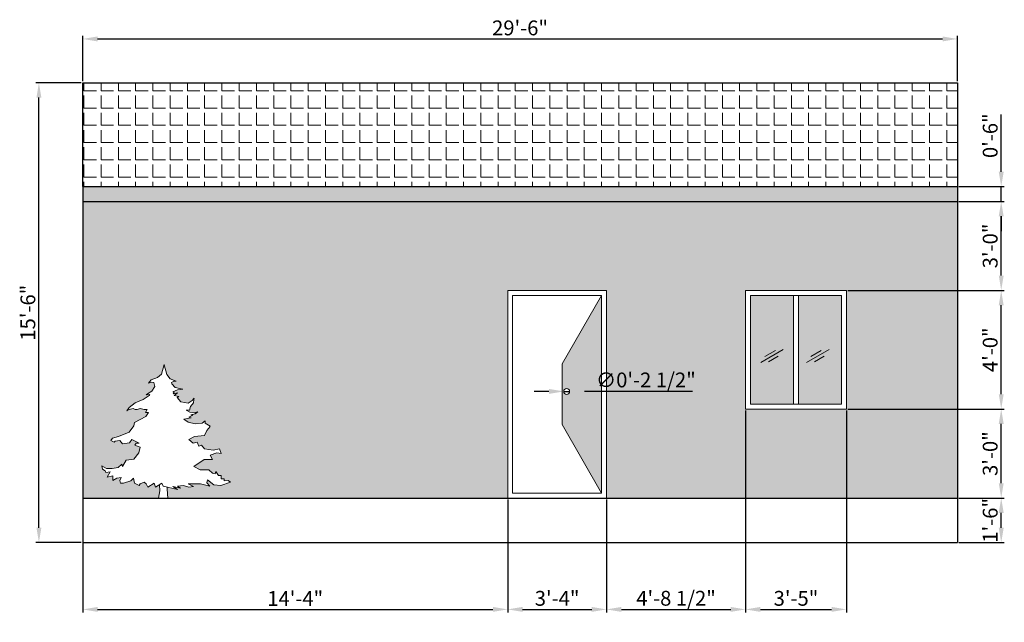
# Model space of a CAD drawing. Units: inches. Extents: x 88375 to 88815, y 24230 to 25146.
# Tile 3 of 3: x 88386 to 88785, y 24902 to 25146. Entities that reach past the tile are written whole.
import ezdxf

# ---------------------------------------------------------------- set-up
doc = ezdxf.new("R2010")
doc.units = ezdxf.units.IN
for name, color, linetype, lineweight in [('A-ANNO-DIMS', 2, 'Continuous', 18), ('A-DOOR-PATT', 34, 'Continuous', 13), ('A-ELEV', 7, 'Continuous', 25), ('doors', 50, 'Continuous', 18), ('L-PLNT', 7, 'Continuous', 13), ('windows', 70, 'Continuous', 18)]:
    doc.layers.add(name, color=color, linetype=linetype, lineweight=lineweight)
for name, color, linetype, lineweight, true_color in [('A-ELEV-PATT', 244, 'Continuous', 13, 0x991b1e), ('A-ELEV-TRIM-PATT', 7, 'Continuous', 13, 0xffffff), ('A-GLAZ-PATT', 141, 'Continuous', 13, 0xadddf7), ('A-ROOF-PATT', 244, 'Continuous', 13, 0x991b1e)]:
    doc.layers.add(name, color=color, linetype=linetype, lineweight=lineweight, true_color=true_color)
doc.styles.get("Standard").update_dxf_attribs({"font": 'arial.ttf'})
doc.dimstyles.new('ISO-25', dxfattribs={"dimtxt": 6, "dimasz": 6, "dimexe": 1.25, "dimexo": 0.625, "dimtad": 1, "dimdec": 0, "dimlunit": 3, "dimtxsty": 'Standard', "dimcen": 2.5, "dimclrd": 1, "dimclre": 1, "dimclrt": 2, "dimadec": 0, "dimazin": 0, "dimtfac": 1, "dimtdec": 0, "dimtmove": 0, "dimatfit": 3, "dimfxl": 1, "dimarcsym": 0})

# ---------------------------------------------------------------- blocks, each defined once
blk = doc.blocks.new('*U7')
for p, q in [((-8.263, 7.598), (-8.747, 14.105)), ((-0.771, 9.56), (-0.69, 11.833)), ((-9.75, 0), (-8.263, 7.598)), ((0, 0), (-0.771, 9.56))]:
    blk.add_line(p, q)
for points in [[(-3.9, 142.35), (-6.596, 132.037), (-10.801, 128.443), (-17.81, 126.047), (-20.614, 122.452), (-17.81, 123.65), (-15.007, 123.051), (-13.605, 118.858), (-16.876, 114.065), (-21.549, 111.07), (-22.951, 109.872), (-19.212, 110.471), (-19.68, 109.273), (-26.222, 105.079), (-34.633, 101.485), (-41.175, 96.693), (-43.511, 93.098), (-41.175, 94.296), (-36.969, 95.494), (-34.633, 94.296), (-32.764, 94.296), (-29.493, 95.494)], [(-3.759, 141.97), (-1.074, 131.643), (2.437, 127.141), (8.84, 124.493), (6.568, 124.493), (4.09, 123.169), (4.296, 121.846), (7.807, 117.874), (16.069, 116.02), (10.492, 115.226), (5.535, 113.372), (6.981, 112.843), (5.948, 110.989), (10.286, 112.048), (6.775, 109.401), (11.732, 108.077), (9.873, 107.282), (13.797, 102.516), (21.852, 101.192), (25.983, 103.84), (28.048, 106.488), (27.842, 105.164), (27.429, 101.457), (24.124, 97.75), (23.091, 93.513), (19.58, 93.513), (23.505, 91.66), (28.255, 90.866), (31.973, 91.925), (29.081, 89.806), (24.537, 88.747), (26.809, 88.218), (22.472, 86.099), (24.95, 85.57), (17.308, 84.246), (21.852, 80.804), (29.081, 79.215), (36.723, 80.009), (39.821, 82.392), (40.028, 80.009), (45.398, 76.567)], [(-29.25, 95.55), (-25.287, 94.296), (-22.016, 94.296), (-23.885, 91.301), (-20.614, 91.301), (-23.418, 87.108), (-35.567, 80.518), (-36.035, 76.924), (-41.175, 70.334), (-52.389, 65.542), (-58.931, 63.744), (-60.8, 61.348), (-57.062, 59.551), (-56.128, 60.749), (-50.987, 61.348), (-48.184, 57.754), (-40.707, 58.952), (-38.371, 62.546), (-30.427, 58.353), (-33.698, 58.353), (-35.1, 56.556), (-29.493, 54.159), (-30.894, 48.169), (-36.035, 41.579), (-44.446, 40.381), (-48.184, 33.791), (-49.118, 36.188), (-52.857, 32.593), (-59.399, 31.395), (-65.473, 31.395), (-70.146, 34.39), (-69.679, 30.796), (-66.875, 28.999), (-65.941, 27.202), (-61.268, 27.801), (-64.539, 22.409), (-58.464, 23.607), (-58.464, 18.815), (-54.258, 21.211), (-49.586, 21.81), (-50.987, 18.815), (-50.52, 15.82), (-47.249, 15.82), (-39.306, 18.216), (-36.502, 21.211), (-35.567, 15.82), (-30.427, 13.423), (-29.493, 15.221), (-25.287, 17.018), (-22.951, 15.221), (-21.081, 11.626), (-14.539, 15.82), (-13.138, 11.626), (-6.128, 15.82), (-4.726, 12.824), (10.226, 9.23), (5.554, 12.225), (13.497, 10.428), (10.226, 12.824), (16.768, 13.423), (22.376, 11.626), (27.516, 12.225), (21.909, 15.221), (34.993, 15.221), (44.806, 12.824), (41.535, 16.419), (42.469, 19.414), (49.011, 14.023), (56.487, 13.423), (66.768, 17.018), (64.431, 18.815), (60.226, 18.216), (60.226, 20.612), (56.955, 20.612), (56.955, 24.206), (54.151, 24.206), (51.348, 28.4), (50.413, 26.004), (47.609, 26.603), (43.871, 30.197), (38.731, 30.197), (34.525, 30.197), (27.983, 33.791), (38.731, 40.98), (47.609, 40.98), (45.273, 45.773), (52.282, 48.169), (56.955, 47.57), (55.086, 52.362), (48.544, 51.164), (39.198, 52.362), (35.927, 56.556), (33.123, 55.357), (31.254, 59.551), (27.049, 58.353), (22.376, 62.546), (28.451, 65.542), (39.198, 66.74), (41.535, 72.131), (45.273, 76.325)]]:
    blk.add_lwpolyline(points)
blk = doc.blocks.new('GLASS-REFLECTION-MARK')
for p, q in [((0, 0), (9.08, 5.24)), ((1.72, 2.48), (5.94, 4.91)), ((3.13, 0.33), (7.04, 2.59))]:
    blk.add_line(p, q)
blk = doc.blocks.new('*D54')
at = {"layer": 'A-ANNO-DIMS', "color": 1, "lineweight": -2, "transparency": 16777216}
for p, q in [((88411.55, 25121.33), (88411.55, 25139.7)), ((88765.55, 25121.33), (88765.55, 25139.7)), ((88417.55, 25138.45), (88759.55, 25138.45))]:
    blk.add_line(p, q, dxfattribs=at)
at = {"layer": 'A-ANNO-DIMS', "color": 1, "transparency": 16777216}
for points in [[(88417.55, 25139.45), (88417.55, 25137.45), (88411.55, 25138.45)], [(88759.55, 25139.45), (88759.55, 25137.45), (88765.55, 25138.45)]]:
    blk.add_solid(points, dxfattribs=at)
at = {"layer": 'Defpoints', "color": 0, "transparency": 16777216}
for p in [(88765.55, 25138.45), (88411.55, 25120.7), (88765.55, 25120.7)]:
    blk.add_point(p, dxfattribs=at)
at = {"layer": 'A-ANNO-DIMS', "color": 2, "transparency": 16777216, "insert": (88588.55, 25142.14), "char_height": 6, "attachment_point": 5}
blk.add_mtext('29\'-6"', dxfattribs=at)
blk = doc.blocks.new('*D55')
at = {"layer": 'A-ANNO-DIMS', "color": 1, "lineweight": -2, "transparency": 16777216}
for p, q in [((88410.93, 25120.7), (88392.55, 25120.7)), ((88393.8, 24940.7), (88393.8, 25114.7)), ((88410.93, 24934.7), (88392.55, 24934.7))]:
    blk.add_line(p, q, dxfattribs=at)
at = {"layer": 'A-ANNO-DIMS', "color": 1, "transparency": 16777216}
for points in [[(88392.8, 25114.7), (88394.8, 25114.7), (88393.8, 25120.7)], [(88392.8, 24940.7), (88394.8, 24940.7), (88393.8, 24934.7)]]:
    blk.add_solid(points, dxfattribs=at)
at = {"layer": 'Defpoints', "color": 0, "transparency": 16777216}
for p in [(88393.8, 25120.7), (88411.55, 25120.7), (88411.55, 24934.7)]:
    blk.add_point(p, dxfattribs=at)
at = {"layer": 'A-ANNO-DIMS', "color": 2, "transparency": 16777216, "insert": (88390.11, 25027.7), "char_height": 6, "attachment_point": 5, "rotation": 90}
blk.add_mtext('15\'-6"', dxfattribs=at)
blk = doc.blocks.new('*D56')
at = {"layer": 'A-ANNO-DIMS', "color": 1, "lineweight": -2, "transparency": 16777216}
for p, q in [((88766.18, 24952.7), (88784.55, 24952.7)), ((88783.3, 24940.7), (88783.3, 24946.7)), ((88766.18, 24934.7), (88784.55, 24934.7))]:
    blk.add_line(p, q, dxfattribs=at)
at = {"layer": 'A-ANNO-DIMS', "color": 1, "transparency": 16777216}
for points in [[(88782.3, 24946.7), (88784.3, 24946.7), (88783.3, 24952.7)], [(88782.3, 24940.7), (88784.3, 24940.7), (88783.3, 24934.7)]]:
    blk.add_solid(points, dxfattribs=at)
at = {"layer": 'Defpoints', "color": 0, "transparency": 16777216}
for p in [(88765.55, 24952.7), (88783.3, 24952.7), (88765.55, 24934.7)]:
    blk.add_point(p, dxfattribs=at)
at = {"layer": 'A-ANNO-DIMS', "color": 2, "transparency": 16777216, "insert": (88779.61, 24943.7), "char_height": 6, "attachment_point": 5, "rotation": 90}
blk.add_mtext('1\'-6"', dxfattribs=at)
blk = doc.blocks.new('*D57')
at = {"layer": 'A-ANNO-DIMS', "color": 1, "lineweight": -2, "transparency": 16777216}
for p, q in [((88766.18, 25072.7), (88784.55, 25072.7)), ((88783.3, 25042.7), (88783.3, 25066.7)), ((88721.25, 25036.7), (88784.55, 25036.7))]:
    blk.add_line(p, q, dxfattribs=at)
at = {"layer": 'A-ANNO-DIMS', "color": 1, "transparency": 16777216}
for points in [[(88782.3, 25066.7), (88784.3, 25066.7), (88783.3, 25072.7)], [(88782.3, 25042.7), (88784.3, 25042.7), (88783.3, 25036.7)]]:
    blk.add_solid(points, dxfattribs=at)
at = {"layer": 'Defpoints', "color": 0, "transparency": 16777216}
for p in [(88765.55, 25072.7), (88783.3, 25072.7), (88720.63, 25036.7)]:
    blk.add_point(p, dxfattribs=at)
at = {"layer": 'A-ANNO-DIMS', "color": 2, "transparency": 16777216, "insert": (88779.61, 25054.7), "char_height": 6, "attachment_point": 5, "rotation": 90}
blk.add_mtext('3\'-0"', dxfattribs=at)
blk = doc.blocks.new('*D58')
at = {"layer": 'A-ANNO-DIMS', "color": 1, "lineweight": -2, "transparency": 16777216}
for p, q in [((88783.3, 25084.7), (88783.3, 25107.9)), ((88766.18, 25078.7), (88784.55, 25078.7)), ((88783.3, 25072.7), (88783.3, 25078.7)), ((88766.18, 25072.7), (88784.55, 25072.7)), ((88783.3, 25066.7), (88783.3, 25060.7))]:
    blk.add_line(p, q, dxfattribs=at)
at = {"layer": 'A-ANNO-DIMS', "color": 1, "transparency": 16777216}
for points in [[(88782.3, 25084.7), (88784.3, 25084.7), (88783.3, 25078.7)], [(88782.3, 25066.7), (88784.3, 25066.7), (88783.3, 25072.7)]]:
    blk.add_solid(points, dxfattribs=at)
at = {"layer": 'Defpoints', "color": 0, "transparency": 16777216}
for p in [(88765.55, 25078.7), (88783.3, 25078.7), (88765.55, 25072.7)]:
    blk.add_point(p, dxfattribs=at)
at = {"layer": 'A-ANNO-DIMS', "color": 2, "transparency": 16777216, "insert": (88779.61, 25099.3), "char_height": 6, "attachment_point": 5, "rotation": 90}
blk.add_mtext('0\'-6"', dxfattribs=at)
blk = doc.blocks.new('*D59')
at = {"layer": 'A-ANNO-DIMS', "color": 1, "lineweight": -2, "transparency": 16777216}
for p, q in [((88411.55, 24952.08), (88411.55, 24906.41)), ((88583.55, 24952.08), (88583.55, 24906.41)), ((88417.55, 24907.66), (88577.55, 24907.66))]:
    blk.add_line(p, q, dxfattribs=at)
at = {"layer": 'A-ANNO-DIMS', "color": 1, "transparency": 16777216}
for points in [[(88417.55, 24908.66), (88417.55, 24906.66), (88411.55, 24907.66)], [(88577.55, 24908.66), (88577.55, 24906.66), (88583.55, 24907.66)]]:
    blk.add_solid(points, dxfattribs=at)
at = {"layer": 'Defpoints', "color": 0, "transparency": 16777216}
for p in [(88411.55, 24952.7), (88583.55, 24952.7), (88583.55, 24907.66)]:
    blk.add_point(p, dxfattribs=at)
at = {"layer": 'A-ANNO-DIMS', "color": 2, "transparency": 16777216, "insert": (88497.55, 24911.3), "char_height": 6, "attachment_point": 5}
blk.add_mtext('14\'-4"', dxfattribs=at)
blk = doc.blocks.new('*D60')
at = {"layer": 'A-ANNO-DIMS', "color": 1, "lineweight": -2, "transparency": 16777216}
for p, q in [((88583.55, 24952.08), (88583.55, 24906.41)), ((88623.55, 24952.08), (88623.55, 24906.41)), ((88589.55, 24907.66), (88617.55, 24907.66))]:
    blk.add_line(p, q, dxfattribs=at)
at = {"layer": 'A-ANNO-DIMS', "color": 1, "transparency": 16777216}
for points in [[(88589.55, 24908.66), (88589.55, 24906.66), (88583.55, 24907.66)], [(88617.55, 24908.66), (88617.55, 24906.66), (88623.55, 24907.66)]]:
    blk.add_solid(points, dxfattribs=at)
at = {"layer": 'Defpoints', "color": 0, "transparency": 16777216}
for p in [(88583.55, 24952.7), (88623.55, 24952.7), (88623.55, 24907.66)]:
    blk.add_point(p, dxfattribs=at)
at = {"layer": 'A-ANNO-DIMS', "color": 2, "transparency": 16777216, "insert": (88603.55, 24911.36), "char_height": 6, "attachment_point": 5}
blk.add_mtext('3\'-4"', dxfattribs=at)
blk = doc.blocks.new('*D61')
at = {"layer": 'A-ANNO-DIMS', "color": 1, "lineweight": -2, "transparency": 16777216}
for p, q in [((88721.25, 24988.7), (88784.55, 24988.7)), ((88783.3, 24958.7), (88783.3, 24982.7)), ((88766.18, 24952.7), (88784.55, 24952.7))]:
    blk.add_line(p, q, dxfattribs=at)
at = {"layer": 'A-ANNO-DIMS', "color": 1, "transparency": 16777216}
for points in [[(88782.3, 24982.7), (88784.3, 24982.7), (88783.3, 24988.7)], [(88782.3, 24958.7), (88784.3, 24958.7), (88783.3, 24952.7)]]:
    blk.add_solid(points, dxfattribs=at)
at = {"layer": 'Defpoints', "color": 0, "transparency": 16777216}
for p in [(88720.63, 24988.7), (88783.3, 24988.7), (88765.55, 24952.7)]:
    blk.add_point(p, dxfattribs=at)
at = {"layer": 'A-ANNO-DIMS', "color": 2, "transparency": 16777216, "insert": (88779.61, 24970.7), "char_height": 6, "attachment_point": 5, "rotation": 90}
blk.add_mtext('3\'-0"', dxfattribs=at)
blk = doc.blocks.new('*D62')
at = {"layer": 'A-ANNO-DIMS', "color": 1, "lineweight": -2, "transparency": 16777216}
for p, q in [((88679.84, 24988.08), (88679.84, 24906.41)), ((88623.55, 24952.08), (88623.55, 24906.41)), ((88629.55, 24907.66), (88673.84, 24907.66))]:
    blk.add_line(p, q, dxfattribs=at)
at = {"layer": 'A-ANNO-DIMS', "color": 1, "transparency": 16777216}
for points in [[(88629.55, 24908.66), (88629.55, 24906.66), (88623.55, 24907.66)], [(88673.84, 24908.66), (88673.84, 24906.66), (88679.84, 24907.66)]]:
    blk.add_solid(points, dxfattribs=at)
at = {"layer": 'Defpoints', "color": 0, "transparency": 16777216}
for p in [(88679.84, 24988.7), (88623.55, 24952.7), (88679.84, 24907.66)]:
    blk.add_point(p, dxfattribs=at)
at = {"layer": 'A-ANNO-DIMS', "color": 2, "transparency": 16777216, "insert": (88651.69, 24911.39), "char_height": 6, "attachment_point": 5}
blk.add_mtext('4\'-8 1/2"', dxfattribs=at)
blk = doc.blocks.new('*D63')
at = {"layer": 'A-ANNO-DIMS', "color": 1, "lineweight": -2, "transparency": 16777216}
for p, q in [((88679.84, 24988.08), (88679.84, 24906.41)), ((88720.63, 24988.08), (88720.63, 24906.41)), ((88685.84, 24907.66), (88714.63, 24907.66))]:
    blk.add_line(p, q, dxfattribs=at)
at = {"layer": 'A-ANNO-DIMS', "color": 1, "transparency": 16777216}
for points in [[(88685.84, 24908.66), (88685.84, 24906.66), (88679.84, 24907.66)], [(88714.63, 24908.66), (88714.63, 24906.66), (88720.63, 24907.66)]]:
    blk.add_solid(points, dxfattribs=at)
at = {"layer": 'Defpoints', "color": 0, "transparency": 16777216}
for p in [(88679.84, 24988.7), (88720.63, 24988.7), (88720.63, 24907.66)]:
    blk.add_point(p, dxfattribs=at)
at = {"layer": 'A-ANNO-DIMS', "color": 2, "transparency": 16777216, "insert": (88700.23, 24911.36), "char_height": 6, "attachment_point": 5}
blk.add_mtext('3\'-5"', dxfattribs=at)
blk = doc.blocks.new('*D64')
at = {"layer": 'A-ANNO-DIMS', "color": 1, "lineweight": -2, "transparency": 16777216}
for p, q in [((88721.25, 25036.7), (88784.55, 25036.7)), ((88783.3, 24994.7), (88783.3, 25030.7)), ((88721.25, 24988.7), (88784.55, 24988.7))]:
    blk.add_line(p, q, dxfattribs=at)
at = {"layer": 'A-ANNO-DIMS', "color": 1, "transparency": 16777216}
for points in [[(88782.3, 25030.7), (88784.3, 25030.7), (88783.3, 25036.7)], [(88782.3, 24994.7), (88784.3, 24994.7), (88783.3, 24988.7)]]:
    blk.add_solid(points, dxfattribs=at)
at = {"layer": 'Defpoints', "color": 0, "transparency": 16777216}
for p in [(88720.63, 25036.7), (88783.3, 25036.7), (88720.63, 24988.7)]:
    blk.add_point(p, dxfattribs=at)
at = {"layer": 'A-ANNO-DIMS', "color": 2, "transparency": 16777216, "insert": (88779.61, 25012.7), "char_height": 6, "attachment_point": 5, "rotation": 90}
blk.add_mtext('4\'-0"', dxfattribs=at)
blk = doc.blocks.new('*D70')
at = {"layer": 'A-ANNO-DIMS', "color": 1, "lineweight": -2, "transparency": 16777216}
for p, q in [((88600.23, 24995.85), (88594.23, 24995.85)), ((88606.23, 24995.85), (88608.61, 24995.85)), ((88658.32, 24995.85), (88614.61, 24995.85))]:
    blk.add_line(p, q, dxfattribs=at)
at = {"layer": 'A-ANNO-DIMS', "color": 1, "transparency": 16777216}
for points in [[(88600.23, 24996.85), (88600.23, 24994.85), (88606.23, 24995.85)], [(88614.61, 24996.85), (88614.61, 24994.85), (88608.61, 24995.85)]]:
    blk.add_solid(points, dxfattribs=at)
at = {"layer": 'Defpoints', "color": 0, "transparency": 16777216}
for p in [(88606.23, 24995.85), (88608.61, 24995.85)]:
    blk.add_point(p, dxfattribs=at)
at = {"layer": 'A-ANNO-DIMS', "color": 2, "transparency": 16777216, "insert": (88639.47, 24999.71), "char_height": 6, "attachment_point": 5, "rotation": 0.0034}
blk.add_mtext('∅0\'-2 1/2"', dxfattribs=at)

msp = doc.modelspace()

# ---------------------------------------------------------------- hatches: boundary and pattern name
at = {"layer": 'A-DOOR-PATT', "transparency": 33554513}
h = msp.add_hatch(color=256, dxfattribs=at)
h.dxf.hatch_style = 1
h.paths.add_polyline_path([(88621.55, 25034.7), (88605.53, 25006.96), (88605.53, 24982.45), (88621.55, 24954.7)])
h.paths.add_polyline_path([(88608.61, 24995.85, -1), (88606.23, 24995.85, -1)], flags=16)
at = {"layer": 'A-ELEV-PATT', "transparency": 33554607}
h = msp.add_hatch(color=256, dxfattribs=at)
h.dxf.hatch_style = 1
h.paths.add_polyline_path([(88583.55, 25036.7), (88623.55, 25036.7), (88623.55, 24952.7), (88765.55, 24952.7), (88765.55, 25072.7), (88411.55, 25072.7), (88411.55, 24952.7), (88442.25, 24952.7), (88442.81, 24955.59), (88442.63, 24958.11), (88440.96, 24957.12), (88440.43, 24958.71), (88437.95, 24957.12), (88437.24, 24958.48), (88436.35, 24959.16), (88434.75, 24958.48), (88434.4, 24957.8), (88432.45, 24958.71), (88432.09, 24960.76), (88431.03, 24959.62), (88428.01, 24958.71), (88426.77, 24958.71), (88426.59, 24959.85), (88427.13, 24960.98), (88425.35, 24960.76), (88423.76, 24959.85), (88423.76, 24961.67), (88421.45, 24961.21), (88422.69, 24963.26), (88420.92, 24963.03), (88420.56, 24963.71), (88419.5, 24964.39), (88419.32, 24965.76), (88421.1, 24964.62), (88423.4, 24964.62), (88425.88, 24965.08), (88427.3, 24966.44), (88427.66, 24965.53), (88429.08, 24968.03), (88432.27, 24968.49), (88434.22, 24970.99), (88434.75, 24973.26), (88432.63, 24974.17), (88433.52, 24975.32), (88431.38, 24976.45), (88430.5, 24975.08), (88427.66, 24974.63), (88426.59, 24975.99), (88424.64, 24975.76), (88424.29, 24975.31), (88422.87, 24975.99), (88423.58, 24976.9), (88426.06, 24977.58), (88430.32, 24979.4), (88432.27, 24981.91), (88432.45, 24983.27), (88437.06, 24985.77), (88438.12, 24987.36), (88436.88, 24987.36), (88437.59, 24988.5), (88436.35, 24988.5), (88434.83, 24988.98), (88433.1, 24988.35), (88431.92, 24988.95), (88430.32, 24988.5), (88429.43, 24988.04), (88430.32, 24989.41), (88432.8, 24991.23), (88436, 24992.59), (88438.48, 24994.19), (88438.66, 24994.64), (88437.24, 24994.41), (88437.77, 24994.87), (88439.54, 24996), (88440.79, 24997.82), (88440.25, 24999.42), (88439.19, 24999.64), (88438.12, 24999.19), (88439.19, 25000.55), (88441.85, 25001.46), (88443.45, 25002.83), (88444.48, 25006.77), (88445.54, 25002.68), (88446.87, 25000.97), (88449.31, 24999.96), (88448.44, 24999.96), (88447.5, 24999.46), (88447.58, 24998.96), (88448.91, 24997.45), (88452.05, 24996.75), (88449.93, 24996.44), (88448.05, 24995.74), (88448.6, 24995.54), (88448.21, 24994.84), (88449.85, 24995.24), (88448.52, 24994.23), (88450.4, 24993.73), (88449.7, 24993.43), (88451.19, 24991.62), (88454.25, 24991.12), (88455.81, 24992.12), (88456.6, 24993.13), (88456.52, 24992.63), (88456.36, 24991.22), (88455.11, 24989.81), (88454.58, 24987.64), (88454.87, 24987.5), (88456.68, 24987.2), (88458.09, 24987.6), (88456.99, 24986.8), (88455.26, 24986.39), (88456.13, 24986.19), (88454.48, 24985.39), (88455.42, 24985.19), (88452.52, 24984.68), (88454.25, 24983.38), (88456.99, 24982.77), (88459.89, 24983.08), (88461.07, 24983.98), (88461.14, 24983.08), (88463.21, 24981.76), (88461.72, 24980.09), (88460.83, 24978.04), (88456.75, 24977.58), (88454.44, 24976.45), (88456.22, 24974.86), (88457.81, 24975.31), (88458.52, 24973.72), (88459.59, 24974.17), (88460.83, 24972.58), (88464.38, 24972.13), (88466.86, 24972.58), (88467.57, 24970.76), (88465.8, 24970.99), (88463.14, 24970.08), (88464.02, 24968.26), (88460.65, 24968.26), (88456.57, 24965.53), (88459.06, 24964.17), (88460.65, 24964.17), (88462.6, 24964.17), (88464.02, 24962.8), (88465.09, 24962.58), (88465.44, 24963.48), (88466.51, 24961.89), (88467.57, 24961.89), (88467.57, 24960.53), (88468.81, 24960.53), (88468.81, 24959.62), (88470.41, 24959.85), (88471.3, 24959.16), (88467.39, 24957.8), (88464.55, 24958.03), (88462.07, 24960.07), (88461.72, 24958.94), (88462.96, 24957.57), (88459.23, 24958.48), (88454.27, 24958.48), (88456.4, 24957.34), (88454.44, 24957.12), (88452.32, 24957.8), (88449.83, 24957.57), (88451.07, 24956.66), (88448.06, 24957.34), (88449.83, 24956.21), (88445.69, 24957.2), (88445.66, 24956.33), (88445.95, 24952.7), (88583.55, 24952.7)])
h.paths.add_polyline_path([(88679.84, 25036.7), (88720.63, 25036.7), (88720.63, 24988.7), (88679.84, 24988.7)], flags=16)
h.paths.add_polyline_path([(88681.84, 25034.7), (88718.63, 25034.7), (88718.63, 24990.7), (88681.84, 24990.7)], flags=0)
h = msp.add_hatch(color=256, dxfattribs=at)
h.dxf.hatch_style = 1
h.paths.add_polyline_path([(88765.55, 25072.7), (88411.55, 25072.7), (88411.55, 24952.7), (88442.25, 24952.7), (88442.81, 24955.59), (88442.63, 24958.11), (88440.96, 24957.12), (88440.43, 24958.71), (88437.95, 24957.12), (88437.24, 24958.48), (88436.35, 24959.16), (88434.75, 24958.48), (88434.4, 24957.8), (88432.45, 24958.71), (88432.09, 24960.76), (88431.03, 24959.62), (88428.01, 24958.71), (88426.77, 24958.71), (88426.59, 24959.85), (88427.13, 24960.98), (88425.35, 24960.76), (88423.76, 24959.85), (88423.76, 24961.67), (88421.45, 24961.21), (88422.69, 24963.26), (88420.92, 24963.03), (88420.56, 24963.71), (88419.5, 24964.39), (88419.32, 24965.76), (88421.1, 24964.62), (88423.4, 24964.62), (88425.88, 24965.08), (88427.3, 24966.44), (88427.66, 24965.53), (88429.08, 24968.03), (88432.27, 24968.49), (88434.22, 24970.99), (88434.75, 24973.26), (88432.63, 24974.17), (88433.52, 24975.32), (88431.38, 24976.45), (88430.5, 24975.08), (88427.66, 24974.63), (88426.59, 24975.99), (88424.64, 24975.76), (88424.29, 24975.31), (88422.87, 24975.99), (88423.58, 24976.9), (88426.06, 24977.58), (88430.32, 24979.4), (88432.27, 24981.91), (88432.45, 24983.27), (88437.06, 24985.77), (88438.12, 24987.36), (88436.88, 24987.36), (88437.59, 24988.5), (88436.35, 24988.5), (88434.83, 24988.98), (88433.1, 24988.35), (88431.92, 24988.95), (88430.32, 24988.5), (88429.43, 24988.04), (88430.32, 24989.41), (88432.8, 24991.23), (88436, 24992.59), (88438.48, 24994.19), (88438.66, 24994.64), (88437.24, 24994.41), (88437.77, 24994.87), (88439.54, 24996), (88440.79, 24997.82), (88440.25, 24999.42), (88439.19, 24999.64), (88438.12, 24999.19), (88439.19, 25000.55), (88441.85, 25001.46), (88443.45, 25002.83), (88444.48, 25006.77), (88445.54, 25002.68), (88446.87, 25000.97), (88449.31, 24999.96), (88448.44, 24999.96), (88447.5, 24999.46), (88447.58, 24998.96), (88448.91, 24997.45), (88452.05, 24996.75), (88449.93, 24996.44), (88448.05, 24995.74), (88448.6, 24995.54), (88448.21, 24994.84), (88449.85, 24995.24), (88448.52, 24994.23), (88450.4, 24993.73), (88449.7, 24993.43), (88451.19, 24991.62), (88454.25, 24991.12), (88455.81, 24992.12), (88456.6, 24993.13), (88456.52, 24992.63), (88456.36, 24991.22), (88455.11, 24989.81), (88454.58, 24987.64), (88454.87, 24987.5), (88456.68, 24987.2), (88458.09, 24987.6), (88456.99, 24986.8), (88455.26, 24986.39), (88456.13, 24986.19), (88454.48, 24985.39), (88455.42, 24985.19), (88452.52, 24984.68), (88454.25, 24983.38), (88456.99, 24982.77), (88459.89, 24983.08), (88461.07, 24983.98), (88461.14, 24983.08), (88463.21, 24981.76), (88461.72, 24980.09), (88460.83, 24978.04), (88456.75, 24977.58), (88454.44, 24976.45), (88456.22, 24974.86), (88457.81, 24975.31), (88458.52, 24973.72), (88459.59, 24974.17), (88460.83, 24972.58), (88464.38, 24972.13), (88466.86, 24972.58), (88467.57, 24970.76), (88465.8, 24970.99), (88463.14, 24970.08), (88464.02, 24968.26), (88460.65, 24968.26), (88456.57, 24965.53), (88459.06, 24964.17), (88460.65, 24964.17), (88462.6, 24964.17), (88464.02, 24962.8), (88465.09, 24962.58), (88465.44, 24963.48), (88466.51, 24961.89), (88467.57, 24961.89), (88467.57, 24960.53), (88468.81, 24960.53), (88468.81, 24959.62), (88470.41, 24959.85), (88471.3, 24959.16), (88467.39, 24957.8), (88464.55, 24958.03), (88462.07, 24960.07), (88461.72, 24958.94), (88462.96, 24957.57), (88459.23, 24958.48), (88454.27, 24958.48), (88456.4, 24957.34), (88454.44, 24957.12), (88452.32, 24957.8), (88449.83, 24957.57), (88451.07, 24956.66), (88448.06, 24957.34), (88449.83, 24956.21), (88445.69, 24957.2), (88445.66, 24956.33), (88445.95, 24952.7), (88583.55, 24952.7), (88583.55, 25036.7), (88623.55, 25036.7), (88623.55, 24952.7), (88765.55, 24952.7)])
h.paths.add_polyline_path([(88679.84, 25036.7), (88720.63, 25036.7), (88720.63, 24988.7), (88679.84, 24988.7)], flags=16)
h.paths.add_polyline_path([(88681.84, 25034.7), (88718.63, 25034.7), (88718.63, 24990.7), (88681.84, 24990.7)], flags=0)
at = {"layer": 'A-ELEV-TRIM-PATT', "transparency": 33554607}
h = msp.add_hatch(color=256, dxfattribs=at)
h.dxf.hatch_style = 1
h.paths.add_polyline_path([(88765.55, 25078.7), (88411.55, 25078.7), (88411.55, 25072.7), (88765.55, 25072.7)])
at = {"layer": 'A-GLAZ-PATT', "transparency": 33554574}
h = msp.add_hatch(color=256, dxfattribs=at)
h.dxf.hatch_style = 1
h.paths.add_polyline_path([(88699.23, 25034.7), (88681.84, 25034.7), (88681.84, 24990.7), (88699.23, 24990.7)])
h.paths.add_polyline_path([(88718.63, 25034.7), (88701.23, 25034.7), (88701.23, 24990.7), (88718.63, 24990.7)])
at = {"layer": 'A-ROOF-PATT'}
h = msp.add_hatch(dxfattribs=at)
h.set_pattern_fill('ANGLE', color=256)
h.set_pattern_definition([(0, (-10027.615, -6762.069), (0, 6.985), [5.08, -1.905]), (90, (-10027.615, -6762.069), (-6.985, 4e-16), [5.08, -1.905])])
h.paths.add_polyline_path([(88765.55, 25120.7), (88411.55, 25120.7), (88411.55, 25078.7), (88765.55, 25078.7)])

# ---------------------------------------------------------------- linework, layer by layer
at = {"layer": 'A-ELEV'}
for p, q in [((88411.55, 25120.7), (88765.55, 25120.7)), ((88411.55, 25078.7), (88411.55, 25120.7)), ((88765.55, 25120.7), (88765.55, 24952.7)), ((88411.55, 25078.7), (88765.55, 25078.7)), ((88411.55, 25078.7), (88411.55, 24952.7)), ((88411.55, 25072.7), (88765.55, 25072.7)), ((88411.55, 24952.7), (88765.55, 24952.7)), ((88411.55, 24952.7), (88411.55, 24934.7)), ((88765.55, 24952.7), (88765.55, 24934.7)), ((88411.55, 24934.7), (88765.55, 24934.7))]:
    msp.add_line(p, q, dxfattribs=at)
at = {"layer": 'doors'}
for p, q in [((88623.55, 24952.7), (88623.55, 25036.7)), ((88621.55, 25034.7), (88605.53, 25006.96)), ((88605.53, 25006.96), (88605.53, 24982.45)), ((88621.55, 24954.7), (88605.53, 24982.45))]:
    msp.add_line(p, q, dxfattribs=at)
for points in [[(88583.55, 24952.7), (88623.55, 24952.7), (88623.55, 25036.7), (88583.55, 25036.7)], [(88585.55, 24954.7), (88621.55, 24954.7), (88621.55, 25034.7), (88585.55, 25034.7)]]:
    msp.add_lwpolyline(points, close=True, dxfattribs=at)
msp.add_circle((88607.42, 24995.85), 1.19, dxfattribs=at)
at = {"layer": 'windows'}
for p, q in [((88699.23, 25034.7), (88699.23, 24990.7)), ((88701.23, 25034.7), (88701.23, 24990.7))]:
    msp.add_line(p, q, dxfattribs=at)
for points in [[(88720.63, 24988.7), (88679.84, 24988.7), (88679.84, 25036.7), (88720.63, 25036.7)], [(88718.63, 24990.7), (88681.84, 24990.7), (88681.84, 25034.7), (88718.63, 25034.7)]]:
    msp.add_lwpolyline(points, close=True, dxfattribs=at)

# ---------------------------------------------------------------- block references
at = {"layer": 'L-PLNT', "xscale": 0.3796093072858473, "yscale": 0.3796093072858473, "zscale": 0.3796093072858473}
msp.add_blockref('*U7', (88445.95, 24952.7), dxfattribs=at)
at = {"layer": 'windows'}
for p in [(88685.96, 25007.55), (88704.54, 25007.55), (88704.54, 25007.55)]:
    msp.add_blockref('GLASS-REFLECTION-MARK', p, dxfattribs=at)

# ---------------------------------------------------------------- dimensions: what is measured, and where the dimension line sits
at = {"layer": 'A-ANNO-DIMS'}
for base, p1, p2, picture, middle in [((88765.55, 25138.45), (88411.55, 25120.7), (88765.55, 25120.7), '*D54', (88588.55, 25142.14)), ((88679.84, 24907.66), (88623.55, 24952.7), (88679.84, 24988.7), '*D62', (88651.69, 24911.39)), ((88720.63, 24907.66), (88679.84, 24988.7), (88720.63, 24988.7), '*D63', (88700.23, 24911.36)), ((88583.55, 24907.66), (88411.55, 24952.7), (88583.55, 24952.7), '*D59', (88497.55, 24911.3)), ((88623.55, 24907.66), (88583.55, 24952.7), (88623.55, 24952.7), '*D60', (88603.55, 24911.36))]:
    dim = msp.add_linear_dim(base=base, p1=p1, p2=p2, dimstyle='ISO-25', override={"dimdec": 1, "dimlfac": 1, "dimrnd": 0, "dimzin": 1, "dimdsep": 46, "dimlunit": 4, "dimfrac": 2}, dxfattribs=at)
    dim.commit()
    dim.dimension.update_dxf_attribs({"geometry": picture, "text_midpoint": middle})
for base, p1, p2, picture, middle in [((88393.8, 25120.7), (88411.55, 24934.7), (88411.55, 25120.7), '*D55', (88390.11, 25027.7)), ((88783.3, 25078.7), (88765.55, 25072.7), (88765.55, 25078.7), '*D58', (88779.61, 25099.3)), ((88783.3, 25072.7), (88720.63, 25036.7), (88765.55, 25072.7), '*D57', (88779.61, 25054.7)), ((88783.3, 25036.7), (88720.63, 24988.7), (88720.63, 25036.7), '*D64', (88779.61, 25012.7)), ((88783.3, 24988.7), (88765.55, 24952.7), (88720.63, 24988.7), '*D61', (88779.61, 24970.7)), ((88783.3, 24952.7), (88765.55, 24934.7), (88765.55, 24952.7), '*D56', (88779.61, 24943.7))]:
    dim = msp.add_linear_dim(base=base, p1=p1, p2=p2, angle=90, dimstyle='ISO-25', override={"dimdec": 1, "dimlfac": 1, "dimrnd": 0, "dimzin": 1, "dimdsep": 46, "dimlunit": 4, "dimfrac": 2}, dxfattribs=at)
    dim.commit()
    dim.dimension.update_dxf_attribs({"geometry": picture, "text_midpoint": middle})
dim = msp.add_diameter_dim_2p(p1=(88606.23, 24995.85), p2=(88608.61, 24995.85), dimstyle='ISO-25', override={"dimdec": 1, "dimlfac": 1, "dimrnd": 0, "dimzin": 1, "dimdsep": 46, "dimlunit": 4, "dimfrac": 2}, dxfattribs=at)
dim.commit()
dim.dimension.update_dxf_attribs({"geometry": '*D70', "text_midpoint": (88639.47, 24995.85)})

doc.saveas('drawing.dxf')
